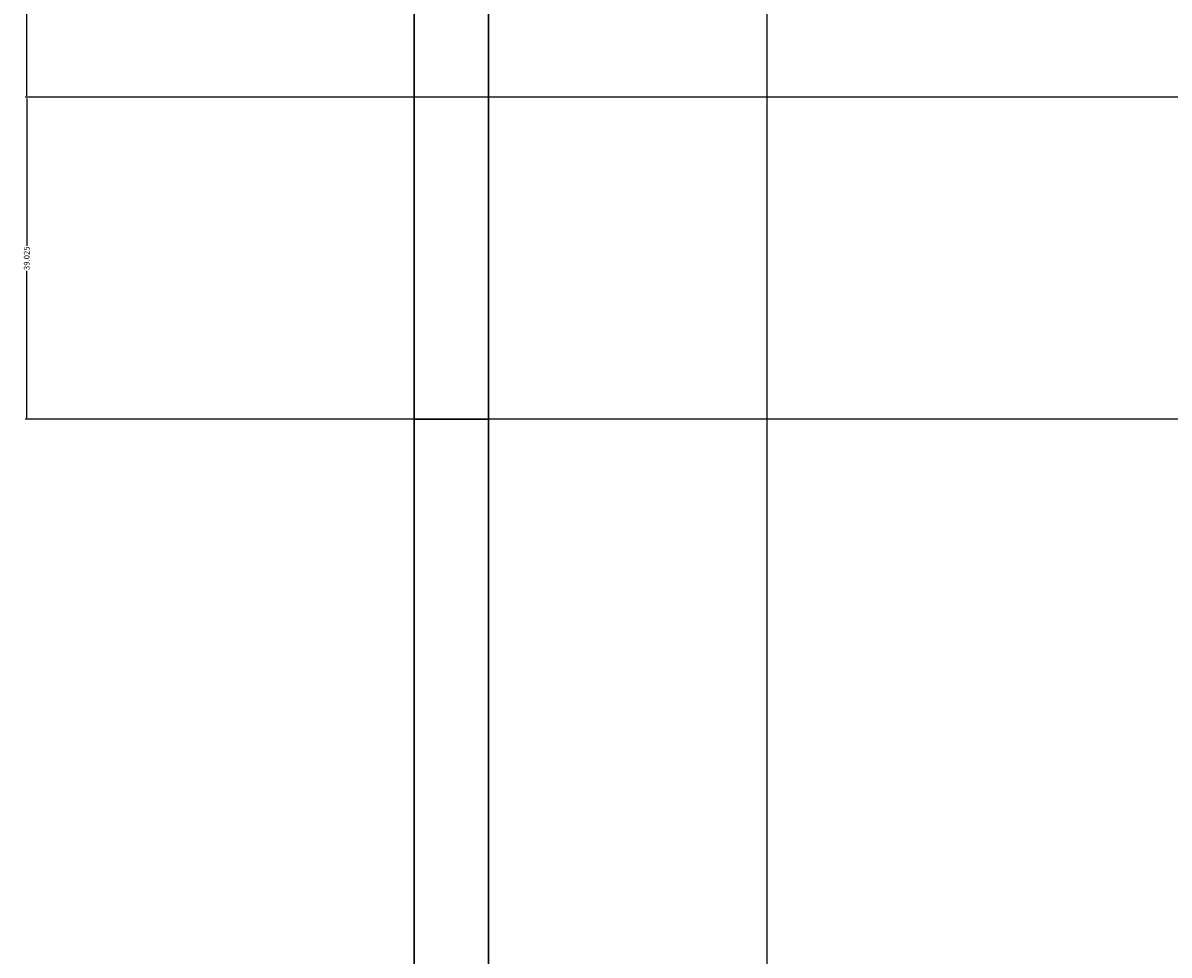
# Model space of a CAD drawing. Units: inches. Extents: x 867 to 1667, y -234 to 788.
# Tile 2 of 42: x 867 to 1006, y -121 to -8. Entities that reach past the tile are written whole.
import ezdxf

# ---------------------------------------------------------------- set-up
doc = ezdxf.new("R2010")
doc.units = ezdxf.units.IN
doc.header["$MEASUREMENT"] = 0
doc.layers.add('A-ANNO-DIMS', color=2, linetype='Continuous', lineweight=18)
doc.layers.add('A-WALL-SITE', color=8, linetype='Continuous', lineweight=30)
doc.styles.get("Standard").update_dxf_attribs({"font": 'arial.ttf'})
doc.dimstyles.get("Standard").update_dxf_attribs({"dimtxt": 0.6875, "dimasz": 0.18, "dimexe": 0.18, "dimexo": 0.0625, "dimgap": 0.09, "dimtad": 0, "dimdec": 4, "dimzin": 0, "dimdsep": 46, "dimlunit": 4, "dimtxsty": 'Standard', "dimcen": 0.09, "dimadec": 0, "dimazin": 0, "dimtfac": 1, "dimtdec": 4, "dimtofl": 0, "dimtmove": 0, "dimatfit": 3, "dimfxl": 1, "dimtolj": 1, "dimtzin": 0, "dimarcsym": 0})

# ---------------------------------------------------------------- blocks, each defined once
blk = doc.blocks.new('*D28')
at = {"layer": 'A-ANNO-DIMS', "color": 0, "lineweight": -2, "transparency": 16777216}
for p, q in [((914.89, 623.55), (914.89, -233.54)), ((957.64, 623.55), (957.64, -233.54)), ((915.07, -233.36), (935, -233.36)), ((957.46, -233.36), (937.53, -233.36))]:
    blk.add_line(p, q, dxfattribs=at)
at = {"layer": 'A-ANNO-DIMS', "color": 0, "transparency": 16777216}
for points in [[(915.07, -233.33), (915.07, -233.39), (914.89, -233.36)], [(957.46, -233.33), (957.46, -233.39), (957.64, -233.36)]]:
    blk.add_solid(points, dxfattribs=at)
at = {"layer": 'Defpoints', "color": 0, "transparency": 16777216}
for p in [(914.89, 623.62), (957.64, 623.62), (914.89, -233.36)]:
    blk.add_point(p, dxfattribs=at)
at = {"layer": 'A-ANNO-DIMS', "color": 0, "transparency": 16777216, "insert": (936.26, -233.36), "char_height": 0.688, "attachment_point": 5}
blk.add_mtext('\\A1;42.75', dxfattribs=at)
blk = doc.blocks.new('*D44')
at = {"layer": 'A-ANNO-DIMS', "color": 0, "lineweight": -2, "transparency": 16777216}
for p, q in [((1070.82, 145.12), (867.76, 145.12)), ((867.94, 144.94), (867.94, 64.93)), ((867.94, -16.7), (867.94, 63.3)), ((1070.82, -16.88), (867.76, -16.88))]:
    blk.add_line(p, q, dxfattribs=at)
at = {"layer": 'A-ANNO-DIMS', "color": 0, "transparency": 16777216}
for points in [[(867.91, 144.94), (867.97, 144.94), (867.94, 145.12)], [(867.91, -16.7), (867.97, -16.7), (867.94, -16.88)]]:
    blk.add_solid(points, dxfattribs=at)
at = {"layer": 'Defpoints', "color": 0, "transparency": 16777216}
for p in [(867.94, 145.12), (1070.89, 145.12), (1070.89, -16.88)]:
    blk.add_point(p, dxfattribs=at)
at = {"layer": 'A-ANNO-DIMS', "color": 0, "transparency": 16777216, "insert": (867.94, 64.12), "char_height": 0.688, "attachment_point": 5, "rotation": 90}
blk.add_mtext('\\A1;162', dxfattribs=at)
blk = doc.blocks.new('*D47')
at = {"layer": 'A-ANNO-DIMS', "color": 0, "lineweight": -2, "transparency": 16777216}
for p, q in [((1070.82, -16.88), (867.76, -16.88)), ((867.94, -17.06), (867.94, -34.88)), ((867.94, -55.73), (867.94, -37.91)), ((1070.82, -55.91), (867.76, -55.91))]:
    blk.add_line(p, q, dxfattribs=at)
at = {"layer": 'A-ANNO-DIMS', "color": 0, "transparency": 16777216}
for points in [[(867.91, -17.06), (867.97, -17.06), (867.94, -16.88)], [(867.91, -55.73), (867.97, -55.73), (867.94, -55.91)]]:
    blk.add_solid(points, dxfattribs=at)
at = {"layer": 'Defpoints', "color": 0, "transparency": 16777216}
for p in [(867.94, -16.88), (1070.89, -16.88), (1070.89, -55.91)]:
    blk.add_point(p, dxfattribs=at)
at = {"layer": 'A-ANNO-DIMS', "color": 0, "transparency": 16777216, "insert": (867.94, -36.4), "char_height": 0.688, "attachment_point": 5, "rotation": 90}
blk.add_mtext('\\A1;39.025', dxfattribs=at)

msp = doc.modelspace()

# ---------------------------------------------------------------- linework, layer by layer
at = {"layer": 'A-WALL-SITE'}
for p, q in [((914.8866, 740.617), (914.8866, -186.4081)), ((923.8866, 740.617), (923.8866, -186.4081)), ((914.8866, -55.9081), (923.8866, -55.9081))]:
    msp.add_line(p, q, dxfattribs=at)

# ---------------------------------------------------------------- dimensions: what is measured, and where the dimension line sits
at = {"layer": 'A-ANNO-DIMS'}
dim = msp.add_linear_dim(base=(914.8866, -233.3581), p1=(957.6375, 623.617), p2=(914.8866, 623.617), dimstyle='Standard', override={"dimdec": 2, "dimlfac": 1, "dimrnd": 0, "dimzin": 0, "dimdsep": 46, "dimlunit": 2}, dxfattribs=at)
dim.commit()
dim.dimension.update_dxf_attribs({"geometry": '*D28', "text_midpoint": (936.2621, -233.3581)})
for base, p1, p2, override, picture, middle in [((867.9366, 145.117), (1070.8866, -16.883), (1070.8866, 145.117), {"dimdec": 0, "dimlfac": 1, "dimrnd": 0, "dimzin": 0, "dimdsep": 46, "dimlunit": 2}, '*D44', (867.9366, 64.117)), ((867.9366, -16.883), (1070.8866, -55.9081), (1070.8866, -16.883), {"dimdec": 3, "dimlfac": 1, "dimrnd": 0, "dimzin": 0, "dimdsep": 46, "dimlunit": 2}, '*D47', (867.9366, -36.3955))]:
    dim = msp.add_linear_dim(base=base, p1=p1, p2=p2, angle=90, dimstyle='Standard', override=override, dxfattribs=at)
    dim.commit()
    dim.dimension.update_dxf_attribs({"geometry": picture, "text_midpoint": middle})

doc.saveas('drawing.dxf')
